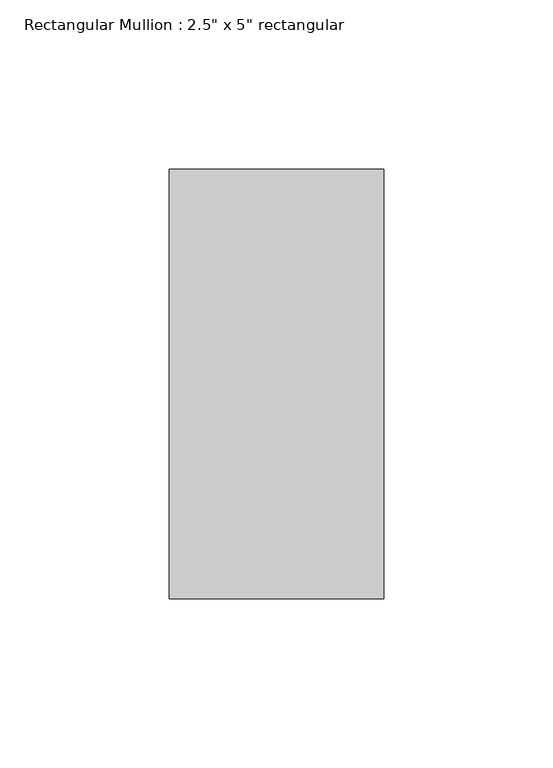
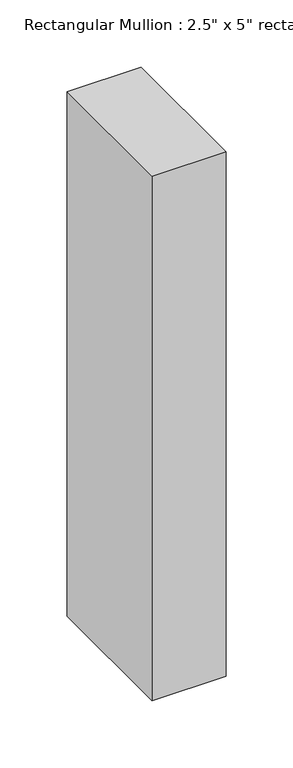
"""IFC4 building model written with IfcOpenShell, lengths in millimetres: member geometry."""

from ifc_helpers import new_model, si_unit, frame, origin, place, context, project, spatial, polyline, outline, extrude, source, transform, mapped, element, save


def member_3728dc7a(model_context):
    return source(origin(), model_context, "Body", "SweptSolid", [
        extrude(outline(polyline([(0.0, 63.5), (0.0, -63.5), (-63.5, -63.5), (-63.5, 63.5), (0.0, 63.5)])), frame((0.0, 0.0, -476.6483121), z_axis=(0.0, 0.0, 1.0), x_axis=(1.0, 0.0, 0.0)), (0.0, 0.0, 1.0), 476.6483121),
    ])


if __name__ == "__main__":
    model = new_model("IFC4")
    model_context = context("Model", 3, world=origin())
    ifc_project = project(units=[si_unit("LENGTHUNIT", "METRE", prefix="MILLI")], contexts=[model_context])
    site = spatial("IfcSite", under=ifc_project)
    building = spatial("IfcBuilding", under=site)
    placement = place(None, origin())
    member_shape = member_3728dc7a(model_context)
    element("IfcMember", 1, ObjectType="Rectangular Mullion : 2.5\" x 5\" rectangular", at=placement, inside=building, context=model_context, shape_type="MappedRepresentation", body=[
        mapped(member_shape, transform((0.0, 0.0, 0.0), x_axis=(1.0, 0.0, 0.0), y_axis=(0.0, 1.0, 0.0), z_axis=(0.0, 0.0, 1.0))),
    ])
    save(model, "model.ifc")

# Revit data of these elements
# Type "Rectangular Mullion : 2.5\" x 5\" rectangular"
#   built-in parameter 1007304 = 0.416667 (stored number, unit not read)
#   built-in parameter 1007301 = 0.104167 (stored number, unit not read)
#   built-in parameter 1007300 = 0.104167 (stored number, unit not read)
# Element 1 (IfcMember, "Rectangular Mullion : 2.5\" x 5\" rectangular")
#   Materials on its faces: "Iron, Ductile"
# Materials
#   "Iron, Ductile": class "Metal", colour RGB 0 0 0, transparency 0, Description = "Ductile cast iron", Cost = 0
